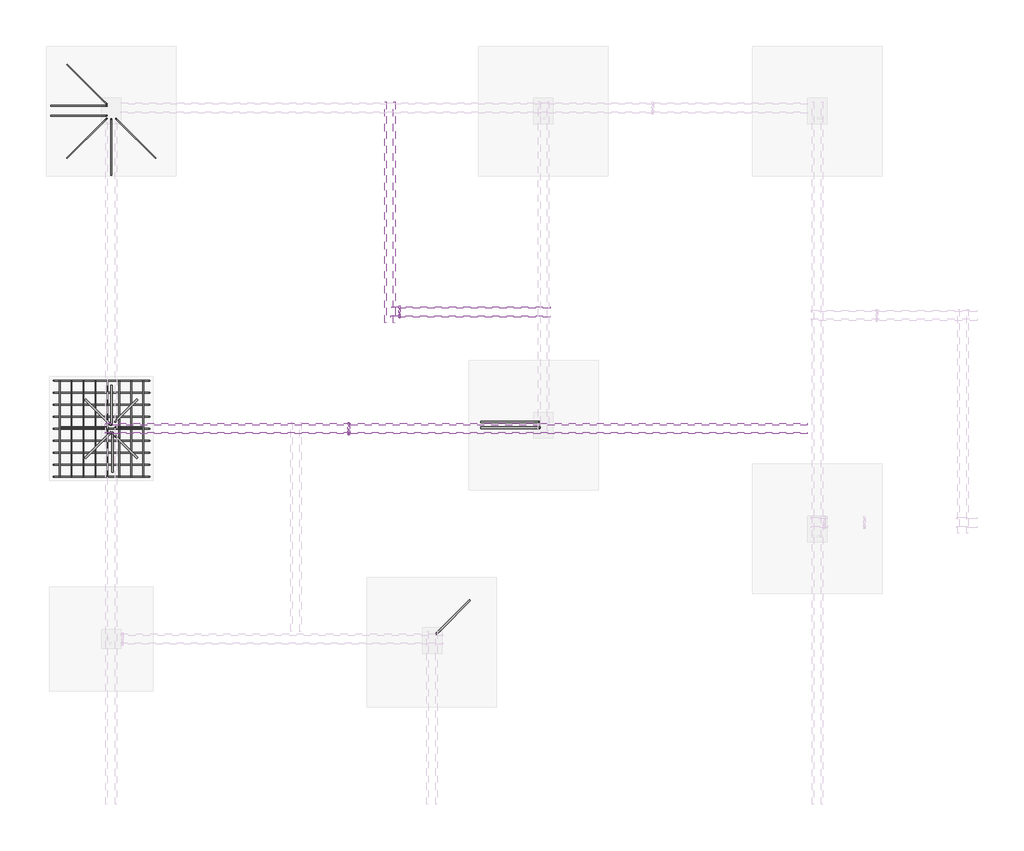
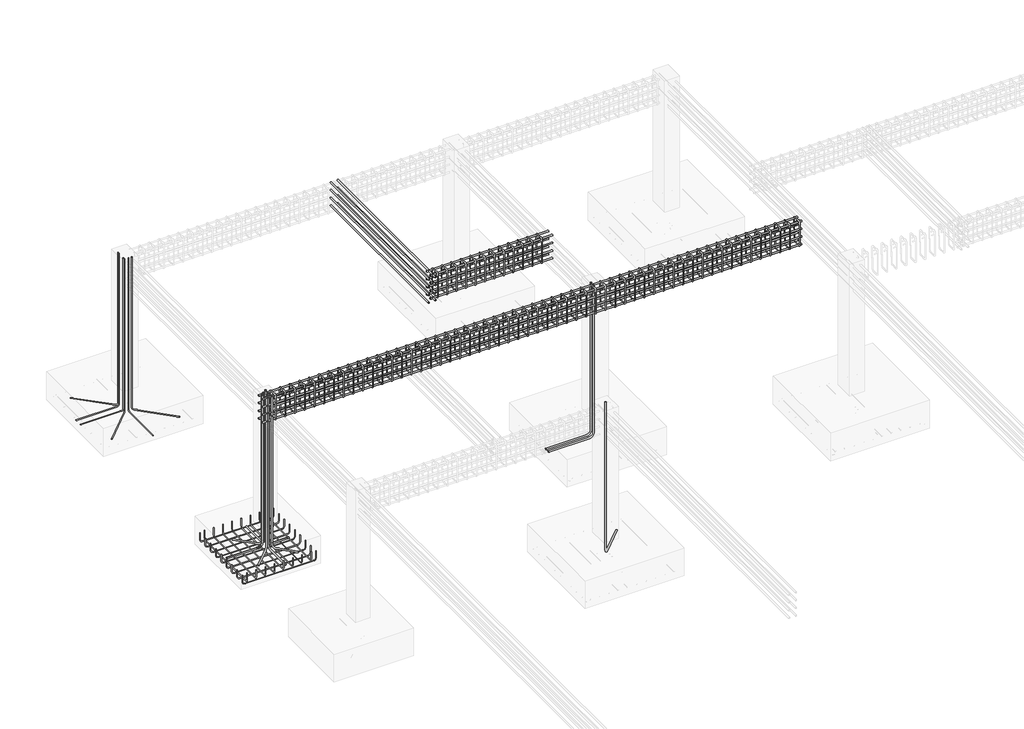
# One storey, part 6 of 10: 28 reinforcing bars.
"""IFC4 building model written with IfcOpenShell, lengths in millimetres."""

from ifc_helpers import new_model, si_unit, point, frame, origin, place, context, project, spatial, polyline, circle_curve, trimmed, segment, composite_curve, source, transform, mapped, element, save
from ifc_brep_helpers import swept_disk

model = new_model("IFC4")

# Units and contexts
model_context = context("Model", 3, world=origin())
ifc_project = project(units=[si_unit("LENGTHUNIT", "METRE", prefix="MILLI")], contexts=[model_context])

# Site, building, storey
site = spatial("IfcSite", under=ifc_project)
building = spatial("IfcBuilding", under=site)
storey = spatial("IfcBuildingStorey", under=building, Elevation=-2133.6)

# Reinforcing bars
placement = place(None, origin())
reinforcing_bar_shape = source(origin(), model_context, "Body", "SolidModel", [
    swept_disk(composite_curve([segment(polyline([(-4484.7164362, 8981.8219177, -2393.6), (-4484.7164362, 8981.8219177, -2504.1)]), True, "CONTINUOUS"), segment(trimmed(circle_curve(frame((-4519.4664362, 8981.8219177, -2504.1), z_axis=(0.0, 1.0, 0.0), x_axis=(34.75, 0.0, 0.0)), 34.75), [point((-4484.7164362, 8981.8219177, -2504.1))], [point((-4519.4664362, 8981.8219177, -2538.85))], True, "CARTESIAN"), True, "CONTINUOUS"), segment(polyline([(-4519.4664362, 8981.8219177, -2538.85), (-5579.6664362, 8981.8219177, -2538.85)]), True, "CONTINUOUS"), segment(trimmed(circle_curve(frame((-5579.6664362, 8981.8219177, -2504.1), z_axis=(0.0, 1.0, 0.0), x_axis=(0.0, 0.0, -34.75)), 34.75), [point((-5579.6664362, 8981.8219177, -2538.85))], [point((-5614.4164362, 8981.8219177, -2504.1))], True, "CARTESIAN"), True, "CONTINUOUS"), segment(polyline([(-5614.4164362, 8981.8219177, -2504.1), (-5614.4164362, 8981.8219177, -2393.6)]), True, "CONTINUOUS")], self_intersect=False), 4.75),
])
element("IfcReinforcingBar", 1, at=placement, inside=storey, context=model_context, shape_type="MappedRepresentation", body=[
    mapped(reinforcing_bar_shape, transform((0.0, 0.0, 0.0), x_axis=(1.0, 0.0, 0.0), y_axis=(0.0, 1.0, 0.0), z_axis=(0.0, 0.0, 1.0))),
    mapped(reinforcing_bar_shape, transform((0.0, -141.2125, 0.0), x_axis=(1.0, 0.0, 0.0), y_axis=(0.0, 1.0, 0.0), z_axis=(0.0, 0.0, 1.0))),
    mapped(reinforcing_bar_shape, transform((0.0, -282.425, 0.0), x_axis=(1.0, 0.0, 0.0), y_axis=(0.0, 1.0, 0.0), z_axis=(0.0, 0.0, 1.0))),
    mapped(reinforcing_bar_shape, transform((0.0, -423.6375, 0.0), x_axis=(1.0, 0.0, 0.0), y_axis=(0.0, 1.0, 0.0), z_axis=(0.0, 0.0, 1.0))),
    mapped(reinforcing_bar_shape, transform((0.0, -564.85, 0.0), x_axis=(1.0, 0.0, 0.0), y_axis=(0.0, 1.0, 0.0), z_axis=(0.0, 0.0, 1.0))),
    mapped(reinforcing_bar_shape, transform((0.0, -706.0625, 0.0), x_axis=(1.0, 0.0, 0.0), y_axis=(0.0, 1.0, 0.0), z_axis=(0.0, 0.0, 1.0))),
    mapped(reinforcing_bar_shape, transform((0.0, -847.275, 0.0), x_axis=(1.0, 0.0, 0.0), y_axis=(0.0, 1.0, 0.0), z_axis=(0.0, 0.0, 1.0))),
    mapped(reinforcing_bar_shape, transform((0.0, -988.4875, 0.0), x_axis=(1.0, 0.0, 0.0), y_axis=(0.0, 1.0, 0.0), z_axis=(0.0, 0.0, 1.0))),
    mapped(reinforcing_bar_shape, transform((0.0, -1129.7, 0.0), x_axis=(1.0, 0.0, 0.0), y_axis=(0.0, 1.0, 0.0), z_axis=(0.0, 0.0, 1.0))),
])
reinforcing_bar_2_shape = source(origin(), model_context, "Body", "SolidModel", [
    swept_disk(composite_curve([segment(polyline([(-4559.6743867, 7852.1219177, -2379.223371), (-4559.6743867, 7852.1219177, -2489.723371)]), True, "CONTINUOUS"), segment(trimmed(circle_curve(frame((-4559.6743867, 7886.8719177, -2489.723371), z_axis=(1.0, 0.0, 0.0), x_axis=(0.0, -34.75, 0.0)), 34.75), [point((-4559.6743867, 7852.1219177, -2489.723371))], [point((-4559.6743867, 7886.8719177, -2524.473371))], True, "CARTESIAN"), True, "CONTINUOUS"), segment(polyline([(-4559.6743867, 7886.8719177, -2524.473371), (-4559.6743867, 8947.0719177, -2524.473371)]), True, "CONTINUOUS"), segment(trimmed(circle_curve(frame((-4559.6743867, 8947.0719177, -2489.723371), z_axis=(1.0, 0.0, 0.0), x_axis=(0.0, 0.0, -34.75)), 34.75), [point((-4559.6743867, 8947.0719177, -2524.473371))], [point((-4559.6743867, 8981.8219177, -2489.723371))], True, "CARTESIAN"), True, "CONTINUOUS"), segment(polyline([(-4559.6743867, 8981.8219177, -2489.723371), (-4559.6743867, 8981.8219177, -2379.223371)]), True, "CONTINUOUS")], self_intersect=False), 4.75),
])
element("IfcReinforcingBar", 2, at=placement, inside=storey, context=model_context, shape_type="MappedRepresentation", body=[
    mapped(reinforcing_bar_2_shape, transform((0.0, 0.0, 0.0), x_axis=(1.0, 0.0, 0.0), y_axis=(0.0, 1.0, 0.0), z_axis=(0.0, 0.0, 1.0))),
    mapped(reinforcing_bar_2_shape, transform((-140.5079612, 0.0, 0.0), x_axis=(1.0, 0.0, 0.0), y_axis=(0.0, 1.0, 0.0), z_axis=(0.0, 0.0, 1.0))),
    mapped(reinforcing_bar_2_shape, transform((-281.0159224, 0.0, 0.0), x_axis=(1.0, 0.0, 0.0), y_axis=(0.0, 1.0, 0.0), z_axis=(0.0, 0.0, 1.0))),
    mapped(reinforcing_bar_2_shape, transform((-421.5238836, 0.0, 0.0), x_axis=(1.0, 0.0, 0.0), y_axis=(0.0, 1.0, 0.0), z_axis=(0.0, 0.0, 1.0))),
    mapped(reinforcing_bar_2_shape, transform((-562.0318448, 0.0, 0.0), x_axis=(1.0, 0.0, 0.0), y_axis=(0.0, 1.0, 0.0), z_axis=(0.0, 0.0, 1.0))),
    mapped(reinforcing_bar_2_shape, transform((-702.539806, 0.0, 0.0), x_axis=(1.0, 0.0, 0.0), y_axis=(0.0, 1.0, 0.0), z_axis=(0.0, 0.0, 1.0))),
    mapped(reinforcing_bar_2_shape, transform((-843.0477672, 0.0, 0.0), x_axis=(1.0, 0.0, 0.0), y_axis=(0.0, 1.0, 0.0), z_axis=(0.0, 0.0, 1.0))),
    mapped(reinforcing_bar_2_shape, transform((-983.5557284, 0.0, 0.0), x_axis=(1.0, 0.0, 0.0), y_axis=(0.0, 1.0, 0.0), z_axis=(0.0, 0.0, 1.0))),
])
element("IfcReinforcingBar", 3, at=placement, inside=storey, context=model_context, shape_type="SolidModel", body=[
    swept_disk(composite_curve([segment(polyline([(-4880.7190942, 12064.1455908, -40.0), (-4880.7190942, 12064.1455908, -2478.85)]), True, "CONTINUOUS"), segment(trimmed(circle_curve(frame((-4856.1471335, 12039.5736302, -2478.85), z_axis=(-0.7071067811865476, -0.7071067811865475, 0.0), x_axis=(-24.57196070000009, 24.57196060000024, 0.0)), 34.75), [point((-4880.7190942, 12064.1455908, -2478.85))], [point((-4856.1471335, 12039.5736302, -2513.6))], True, "CARTESIAN"), True, "CONTINUOUS"), segment(polyline([(-4856.1471335, 12039.5736302, -2513.6), (-4415.8298614, 11599.256358, -2513.6)]), True, "CONTINUOUS")], self_intersect=False), 4.75),
])
element("IfcReinforcingBar", 4, at=placement, inside=storey, context=model_context, shape_type="SolidModel", body=[
    swept_disk(composite_curve([segment(polyline([(-4989.8137781, 12064.1455908, -40.0), (-4989.8137781, 12064.1455908, -2478.85)]), True, "CONTINUOUS"), segment(trimmed(circle_curve(frame((-5014.3857388, 12039.5736302, -2478.85), z_axis=(-0.7071067811865476, 0.7071067811865475, 0.0), x_axis=(24.57196070000009, 24.57196060000024, 0.0)), 34.75), [point((-4989.8137781, 12064.1455908, -2478.85))], [point((-5014.3857388, 12039.5736302, -2513.6))], True, "CARTESIAN"), True, "CONTINUOUS"), segment(polyline([(-5014.3857388, 12039.5736302, -2513.6), (-5454.7030109, 11599.256358, -2513.6)]), True, "CONTINUOUS")], self_intersect=False), 4.75),
])
element("IfcReinforcingBar", 5, at=placement, inside=storey, context=model_context, shape_type="SolidModel", body=[
    swept_disk(composite_curve([segment(polyline([(-4989.8137781, 12237.3982446, -40.0), (-4989.8137781, 12237.3982446, -2478.85)]), True, "CONTINUOUS"), segment(trimmed(circle_curve(frame((-5014.3857388, 12261.9702053, -2478.85), z_axis=(0.7071067811865476, 0.7071067811865475, 0.0), x_axis=(24.57196070000009, -24.57196069999918, 0.0)), 34.75), [point((-4989.8137781, 12237.3982446, -2478.85))], [point((-5014.3857388, 12261.9702053, -2513.6))], True, "CARTESIAN"), True, "CONTINUOUS"), segment(polyline([(-5014.3857388, 12261.9702053, -2513.6), (-5454.7030109, 12702.2874774, -2513.6)]), True, "CONTINUOUS")], self_intersect=False), 4.75),
])
reinforcing_bar_3_shape = source(origin(), model_context, "Body", "SolidModel", [
    swept_disk(composite_curve([segment(polyline([(-4989.8137781, 12214.7595351, -40.0), (-4989.8137781, 12214.7595351, -2478.85)]), True, "CONTINUOUS"), segment(trimmed(circle_curve(frame((-5024.5637781, 12214.7595351, -2478.85), z_axis=(0.0, 1.0, 0.0), x_axis=(34.75, 0.0, 0.0)), 34.75), [point((-4989.8137781, 12214.7595351, -2478.85))], [point((-5024.5637781, 12214.7595351, -2513.6))], True, "CARTESIAN"), True, "CONTINUOUS"), segment(polyline([(-5024.5637781, 12214.7595351, -2513.6), (-5647.2664362, 12214.7595351, -2513.6)]), True, "CONTINUOUS")], self_intersect=False), 4.75),
])
element("IfcReinforcingBar", 6, at=placement, inside=storey, context=model_context, shape_type="MappedRepresentation", body=[
    mapped(reinforcing_bar_3_shape, transform((0.0, 0.0, 0.0), x_axis=(1.0, 0.0, 0.0), y_axis=(0.0, 1.0, 0.0), z_axis=(0.0, 0.0, 1.0))),
    mapped(reinforcing_bar_3_shape, transform((0.0, -114.7595265, 0.0), x_axis=(1.0, 0.0, 0.0), y_axis=(0.0, 1.0, 0.0), z_axis=(0.0, 0.0, 1.0))),
])
element("IfcReinforcingBar", 7, at=placement, inside=storey, context=model_context, shape_type="SolidModel", body=[
    swept_disk(composite_curve([segment(polyline([(-4935.2664362, 12059.1455908, -40.0), (-4935.2664362, 12059.1455908, -2478.85)]), True, "CONTINUOUS"), segment(trimmed(circle_curve(frame((-4935.2664362, 12024.3955908, -2478.85), z_axis=(-1.0, 0.0, 0.0), x_axis=(0.0, 34.75, 0.0)), 34.75), [point((-4935.2664362, 12059.1455908, -2478.85))], [point((-4935.2664362, 12024.3955908, -2513.6))], True, "CARTESIAN"), True, "CONTINUOUS"), segment(polyline([(-4935.2664362, 12024.3955908, -2513.6), (-4935.2664362, 11401.6929328, -2513.6)]), True, "CONTINUOUS")], self_intersect=False), 4.75),
])
element("IfcReinforcingBar", 8, at=placement, inside=storey, context=model_context, shape_type="SolidModel", body=[
    swept_disk(composite_curve([segment(polyline([(103.8835638, 8496.2552961, -40.0), (103.8835638, 8496.2552961, -2426.55)]), True, "CONTINUOUS"), segment(trimmed(circle_curve(frame((36.8335638, 8496.2552961, -2426.55), z_axis=(0.0, 1.0, 0.0), x_axis=(67.05000000000001, 0.0, 0.0)), 67.05), [point((103.8835638, 8496.2552961, -2426.55))], [point((36.8335638, 8496.2552961, -2493.6))], True, "CARTESIAN"), True, "CONTINUOUS"), segment(polyline([(36.8335638, 8496.2552961, -2493.6), (-590.4164362, 8496.2552961, -2493.6)]), True, "CONTINUOUS")], self_intersect=False), 9.55),
])
element("IfcReinforcingBar", 9, at=placement, inside=storey, context=model_context, shape_type="SolidModel", body=[
    swept_disk(composite_curve([segment(polyline([(103.8835638, 8429.1170998, -40.0), (103.8835638, 8429.1170998, -2426.55)]), True, "CONTINUOUS"), segment(trimmed(circle_curve(frame((36.8335638, 8429.1170998, -2426.55), z_axis=(0.0, 1.0, 0.0), x_axis=(67.05000000000001, 0.0, 0.0)), 67.05), [point((103.8835638, 8429.1170998, -2426.55))], [point((36.8335638, 8429.1170998, -2493.6))], True, "CARTESIAN"), True, "CONTINUOUS"), segment(polyline([(36.8335638, 8429.1170998, -2493.6), (-590.4164362, 8429.1170998, -2493.6)]), True, "CONTINUOUS")], self_intersect=False), 9.55),
])
element("IfcReinforcingBar", 10, at=placement, inside=storey, context=model_context, shape_type="SolidModel", body=[
    swept_disk(composite_curve([segment(polyline([(-4944.3664362, 8465.0552961, -40.0), (-4944.3664362, 8465.0552961, -2426.55)]), True, "CONTINUOUS"), segment(trimmed(circle_curve(frame((-4991.7779458, 8512.4668058, -2426.55), z_axis=(0.7071067811865519, 0.7071067811865431, 0.0), x_axis=(47.4115096000005, -47.41150970000126, 0.0)), 67.05), [point((-4944.3664362, 8465.0552961, -2426.55))], [point((-4991.7779458, 8512.4668058, -2493.6))], True, "CARTESIAN"), True, "CONTINUOUS"), segment(polyline([(-4991.7779458, 8512.4668058, -2493.6), (-5240.1883692, 8760.8772292, -2493.6)]), True, "CONTINUOUS")], self_intersect=False), 9.55),
])
element("IfcReinforcingBar", 11, at=placement, inside=storey, context=model_context, shape_type="SolidModel", body=[
    swept_disk(composite_curve([segment(polyline([(-4886.9664362, 8503.1552961, -40.0), (-4886.9664362, 8503.1552961, -2426.55)]), True, "CONTINUOUS"), segment(trimmed(circle_curve(frame((-4839.5549265, 8550.5668058, -2426.55), z_axis=(0.7071067811865519, -0.7071067811865431, 0.0), x_axis=(-47.41150970000035, -47.41150969999944, 0.0)), 67.05), [point((-4886.9664362, 8503.1552961, -2426.55))], [point((-4839.5549265, 8550.5668058, -2493.6))], True, "CARTESIAN"), True, "CONTINUOUS"), segment(polyline([(-4839.5549265, 8550.5668058, -2493.6), (-4629.2445031, 8760.8772292, -2493.6)]), True, "CONTINUOUS")], self_intersect=False), 9.55),
])
element("IfcReinforcingBar", 12, at=placement, inside=storey, context=model_context, shape_type="SolidModel", body=[
    swept_disk(composite_curve([segment(polyline([(-4944.3664362, 8368.8885393, -40.0), (-4944.3664362, 8368.8885393, -2426.55)]), True, "CONTINUOUS"), segment(trimmed(circle_curve(frame((-4991.7779458, 8321.4770296, -2426.55), z_axis=(-0.7071067811865519, 0.7071067811865431, 0.0), x_axis=(47.4115096000005, 47.41150969999944, 0.0)), 67.05), [point((-4944.3664362, 8368.8885393, -2426.55))], [point((-4991.7779458, 8321.4770296, -2493.6))], True, "CARTESIAN"), True, "CONTINUOUS"), segment(polyline([(-4991.7779458, 8321.4770296, -2493.6), (-5240.1883692, 8073.0666062, -2493.6)]), True, "CONTINUOUS")], self_intersect=False), 9.55),
])
element("IfcReinforcingBar", 13, at=placement, inside=storey, context=model_context, shape_type="SolidModel", body=[
    swept_disk(composite_curve([segment(polyline([(-4886.9664362, 8330.7885393, -40.0), (-4886.9664362, 8330.7885393, -2426.55)]), True, "CONTINUOUS"), segment(trimmed(circle_curve(frame((-4839.5549265, 8283.3770296, -2426.55), z_axis=(-0.7071067811865519, -0.7071067811865431, 0.0), x_axis=(-47.41150970000035, 47.41150969999944, 0.0)), 67.05), [point((-4886.9664362, 8330.7885393, -2426.55))], [point((-4839.5549265, 8283.3770296, -2493.6))], True, "CARTESIAN"), True, "CONTINUOUS"), segment(polyline([(-4839.5549265, 8283.3770296, -2493.6), (-4629.2445031, 8073.0666062, -2493.6)]), True, "CONTINUOUS")], self_intersect=False), 9.55),
])
element("IfcReinforcingBar", 14, at=placement, inside=storey, context=model_context, shape_type="SolidModel", body=[
    swept_disk(composite_curve([segment(polyline([(-4933.5805145, 8465.0552961, -40.0), (-4933.5805145, 8465.0552961, -2426.55)]), True, "CONTINUOUS"), segment(trimmed(circle_curve(frame((-4933.5805145, 8532.1052961, -2426.55), z_axis=(1.0, 0.0, 0.0), x_axis=(0.0, -67.05000000000109, 0.0)), 67.05), [point((-4933.5805145, 8465.0552961, -2426.55))], [point((-4933.5805145, 8532.1052961, -2493.6))], True, "CARTESIAN"), True, "CONTINUOUS"), segment(polyline([(-4933.5805145, 8532.1052961, -2493.6), (-4933.5805145, 8930.7552961, -2493.6)]), True, "CONTINUOUS")], self_intersect=False), 9.55),
])
element("IfcReinforcingBar", 15, at=placement, inside=storey, context=model_context, shape_type="SolidModel", body=[
    swept_disk(composite_curve([segment(polyline([(-4923.5805145, 8368.8885393, -40.0), (-4923.5805145, 8368.8885393, -2426.55)]), True, "CONTINUOUS"), segment(trimmed(circle_curve(frame((-4923.5805145, 8301.8385393, -2426.55), z_axis=(-1.0, 0.0, 0.0), x_axis=(0.0, 67.04999999999927, 0.0)), 67.05), [point((-4923.5805145, 8368.8885393, -2426.55))], [point((-4923.5805145, 8301.8385393, -2493.6))], True, "CARTESIAN"), True, "CONTINUOUS"), segment(polyline([(-4923.5805145, 8301.8385393, -2493.6), (-4923.5805145, 7903.1885393, -2493.6)]), True, "CONTINUOUS")], self_intersect=False), 9.55),
])
element("IfcReinforcingBar", 16, at=placement, inside=storey, context=model_context, shape_type="SolidModel", body=[
    swept_disk(composite_curve([segment(polyline([(-4982.4664362, 8420.0552961, -40.0), (-4982.4664362, 8420.0552961, -2426.55)]), True, "CONTINUOUS"), segment(trimmed(circle_curve(frame((-5049.5164362, 8420.0552961, -2426.55), z_axis=(0.0, 1.0, 0.0), x_axis=(67.04999999999927, 0.0, 0.0)), 67.05), [point((-4982.4664362, 8420.0552961, -2426.55))], [point((-5049.5164362, 8420.0552961, -2493.6))], True, "CARTESIAN"), True, "CONTINUOUS"), segment(polyline([(-5049.5164362, 8420.0552961, -2493.6), (-5524.3664362, 8420.0552961, -2493.6)]), True, "CONTINUOUS")], self_intersect=False), 9.55),
])
element("IfcReinforcingBar", 17, at=placement, inside=storey, context=model_context, shape_type="SolidModel", body=[
    swept_disk(composite_curve([segment(polyline([(-4982.4664362, 8429.1170998, -40.0), (-4982.4664362, 8429.1170998, -2426.55)]), True, "CONTINUOUS"), segment(trimmed(circle_curve(frame((-5049.5164362, 8429.1170998, -2426.55), z_axis=(0.0, 1.0, 0.0), x_axis=(67.04999999999927, 0.0, 0.0)), 67.05), [point((-4982.4664362, 8429.1170998, -2426.55))], [point((-5049.5164362, 8429.1170998, -2493.6))], True, "CARTESIAN"), True, "CONTINUOUS"), segment(polyline([(-5049.5164362, 8429.1170998, -2493.6), (-5524.3664362, 8429.1170998, -2493.6)]), True, "CONTINUOUS")], self_intersect=False), 9.55),
])
element("IfcReinforcingBar", 18, at=placement, inside=storey, context=model_context, shape_type="SolidModel", body=[
    swept_disk(composite_curve([segment(polyline([(-4886.9664362, 8420.0552961, -40.0), (-4886.9664362, 8420.0552961, -2426.55)]), True, "CONTINUOUS"), segment(trimmed(circle_curve(frame((-4819.9164362, 8420.0552961, -2426.55), z_axis=(0.0, -1.0, 0.0), x_axis=(-67.05000000000018, 0.0, 0.0)), 67.05), [point((-4886.9664362, 8420.0552961, -2426.55))], [point((-4819.9164362, 8420.0552961, -2493.6))], True, "CARTESIAN"), True, "CONTINUOUS"), segment(polyline([(-4819.9164362, 8420.0552961, -2493.6), (-4573.6664362, 8420.0552961, -2493.6)]), True, "CONTINUOUS")], self_intersect=False), 9.55),
])
element("IfcReinforcingBar", 19, at=placement, inside=storey, context=model_context, shape_type="SolidModel", body=[
    swept_disk(composite_curve([segment(polyline([(-4886.9664362, 8429.1170998, -40.0), (-4886.9664362, 8429.1170998, -2426.55)]), True, "CONTINUOUS"), segment(trimmed(circle_curve(frame((-4819.9164362, 8429.1170998, -2426.55), z_axis=(0.0, -1.0, 0.0), x_axis=(-67.05000000000018, 0.0, 0.0)), 67.05), [point((-4886.9664362, 8429.1170998, -2426.55))], [point((-4819.9164362, 8429.1170998, -2493.6))], True, "CARTESIAN"), True, "CONTINUOUS"), segment(polyline([(-4819.9164362, 8429.1170998, -2493.6), (-4573.6664362, 8429.1170998, -2493.6)]), True, "CONTINUOUS")], self_intersect=False), 9.55),
])
element("IfcReinforcingBar", 20, at=placement, inside=storey, context=model_context, shape_type="SolidModel", body=[
    swept_disk(composite_curve([segment(polyline([(-1109.9664362, 6006.6552961, -40.0), (-1109.9664362, 6006.6552961, -2426.55)]), True, "CONTINUOUS"), segment(trimmed(circle_curve(frame((-1062.5549265, 6054.0668058, -2426.55), z_axis=(0.7071067811865519, -0.7071067811865431, 0.0), x_axis=(-47.411509700000124, -47.41150970000035, 0.0)), 67.05), [point((-1109.9664362, 6006.6552961, -2426.55))], [point((-1062.5549265, 6054.0668058, -2493.6))], True, "CARTESIAN"), True, "CONTINUOUS"), segment(polyline([(-1062.5549265, 6054.0668058, -2493.6), (-717.9445031, 6398.6772292, -2493.6)]), True, "CONTINUOUS")], self_intersect=False), 9.55),
])
reinforcing_bar_4_shape = source(origin(), model_context, "Body", "SolidModel", [
    swept_disk(composite_curve([segment(polyline([(-4816.2164362, 8447.0786993, -109.4049959), (-4816.2164362, 8389.6728105, -51.9991072)]), True, "CONTINUOUS"), segment(trimmed(circle_curve(frame((-4816.2164362, 8372.1719177, -69.5), z_axis=(1.0, 0.0, 0.0), x_axis=(0.0, 17.500892800000656, 17.500892800000003)), 24.75), [point((-4816.2164362, 8389.6728105, -51.9991072))], [point((-4816.2164362, 8347.4219177, -69.5))], True, "CARTESIAN"), True, "CONTINUOUS"), segment(polyline([(-4816.2164362, 8347.4219177, -69.5), (-4816.2164362, 8347.4219177, -430.5)]), True, "CONTINUOUS"), segment(trimmed(circle_curve(frame((-4816.2164362, 8372.1719177, -430.5), z_axis=(1.0, 0.0, 0.0), x_axis=(0.0, -24.75, 0.0)), 24.75), [point((-4816.2164362, 8347.4219177, -430.5))], [point((-4816.2164362, 8372.1719177, -455.25))], True, "CARTESIAN"), True, "CONTINUOUS"), segment(polyline([(-4816.2164362, 8372.1719177, -455.25), (-4816.2164362, 8461.7719177, -455.25)]), True, "CONTINUOUS"), segment(trimmed(circle_curve(frame((-4816.7890599, 8461.7719177, -430.5066251), z_axis=(0.9997323196529888, 0.0, 0.02313631434032496), x_axis=(0.5726236999998946, 0.0, -24.743374899999992)), 24.75), [point((-4816.2164362, 8461.7719177, -455.25))], [point((-4816.7890599, 8486.5219177, -430.5066251))], True, "CARTESIAN"), True, "CONTINUOUS"), segment(polyline([(-4816.7890599, 8486.5219177, -430.5066251), (-4825.1438124, 8486.5219177, -69.4933749)]), True, "CONTINUOUS"), segment(trimmed(circle_curve(frame((-4825.1438124, 8461.7719177, -69.4933749), z_axis=(0.9997323196529888, 0.0, 0.02313631434032496), x_axis=(0.0, 24.75, 0.0)), 24.75), [point((-4825.1438124, 8486.5219177, -69.4933749))], [point((-4825.7164362, 8461.7719177, -44.75))], True, "CARTESIAN"), True, "CONTINUOUS"), segment(polyline([(-4825.7164362, 8461.7719177, -44.75), (-4825.7164362, 8372.1719177, -44.75)]), True, "CONTINUOUS"), segment(trimmed(circle_curve(frame((-4825.7164362, 8372.1719177, -69.5), z_axis=(1.0, 0.0, 0.0), x_axis=(0.0, 0.0, 24.75)), 24.75), [point((-4825.7164362, 8372.1719177, -44.75))], [point((-4825.7164362, 8354.6710249, -87.0008928))], True, "CARTESIAN"), True, "CONTINUOUS"), segment(polyline([(-4825.7164362, 8354.6710249, -87.0008928), (-4825.7164362, 8412.0769136, -144.4067815)]), True, "CONTINUOUS")], self_intersect=False), 4.75),
])
element("IfcReinforcingBar", 21, at=placement, inside=storey, context=model_context, shape_type="MappedRepresentation", body=[
    mapped(reinforcing_bar_4_shape, transform((0.0, 0.0, 0.0), x_axis=(1.0, 0.0, 0.0), y_axis=(0.0, 1.0, 0.0), z_axis=(0.0, 0.0, 1.0))),
    mapped(reinforcing_bar_4_shape, transform((148.8172337, 0.0, 0.0), x_axis=(1.0, 0.0, 0.0), y_axis=(0.0, 1.0, 0.0), z_axis=(0.0, 0.0, 1.0))),
    mapped(reinforcing_bar_4_shape, transform((297.6344674, 0.0, 0.0), x_axis=(1.0, 0.0, 0.0), y_axis=(0.0, 1.0, 0.0), z_axis=(0.0, 0.0, 1.0))),
    mapped(reinforcing_bar_4_shape, transform((446.4517011, 0.0, 0.0), x_axis=(1.0, 0.0, 0.0), y_axis=(0.0, 1.0, 0.0), z_axis=(0.0, 0.0, 1.0))),
    mapped(reinforcing_bar_4_shape, transform((595.2689349, 0.0, 0.0), x_axis=(1.0, 0.0, 0.0), y_axis=(0.0, 1.0, 0.0), z_axis=(0.0, 0.0, 1.0))),
    mapped(reinforcing_bar_4_shape, transform((744.0861686, 0.0, 0.0), x_axis=(1.0, 0.0, 0.0), y_axis=(0.0, 1.0, 0.0), z_axis=(0.0, 0.0, 1.0))),
    mapped(reinforcing_bar_4_shape, transform((892.9034023, 0.0, 0.0), x_axis=(1.0, 0.0, 0.0), y_axis=(0.0, 1.0, 0.0), z_axis=(0.0, 0.0, 1.0))),
    mapped(reinforcing_bar_4_shape, transform((1041.720636, 0.0, 0.0), x_axis=(1.0, 0.0, 0.0), y_axis=(0.0, 1.0, 0.0), z_axis=(0.0, 0.0, 1.0))),
    mapped(reinforcing_bar_4_shape, transform((1190.5378697, 0.0, 0.0), x_axis=(1.0, 0.0, 0.0), y_axis=(0.0, 1.0, 0.0), z_axis=(0.0, 0.0, 1.0))),
    mapped(reinforcing_bar_4_shape, transform((1339.3551034, 0.0, 0.0), x_axis=(1.0, 0.0, 0.0), y_axis=(0.0, 1.0, 0.0), z_axis=(0.0, 0.0, 1.0))),
    mapped(reinforcing_bar_4_shape, transform((1488.1723371, 0.0, 0.0), x_axis=(1.0, 0.0, 0.0), y_axis=(0.0, 1.0, 0.0), z_axis=(0.0, 0.0, 1.0))),
    mapped(reinforcing_bar_4_shape, transform((1636.9895708, 0.0, 0.0), x_axis=(1.0, 0.0, 0.0), y_axis=(0.0, 1.0, 0.0), z_axis=(0.0, 0.0, 1.0))),
    mapped(reinforcing_bar_4_shape, transform((1785.8068046, 0.0, 0.0), x_axis=(1.0, 0.0, 0.0), y_axis=(0.0, 1.0, 0.0), z_axis=(0.0, 0.0, 1.0))),
    mapped(reinforcing_bar_4_shape, transform((1934.6240383, 0.0, 0.0), x_axis=(1.0, 0.0, 0.0), y_axis=(0.0, 1.0, 0.0), z_axis=(0.0, 0.0, 1.0))),
    mapped(reinforcing_bar_4_shape, transform((2083.441272, 0.0, 0.0), x_axis=(1.0, 0.0, 0.0), y_axis=(0.0, 1.0, 0.0), z_axis=(0.0, 0.0, 1.0))),
    mapped(reinforcing_bar_4_shape, transform((2232.2585057, 0.0, 0.0), x_axis=(1.0, 0.0, 0.0), y_axis=(0.0, 1.0, 0.0), z_axis=(0.0, 0.0, 1.0))),
    mapped(reinforcing_bar_4_shape, transform((2381.0757394, 0.0, 0.0), x_axis=(1.0, 0.0, 0.0), y_axis=(0.0, 1.0, 0.0), z_axis=(0.0, 0.0, 1.0))),
    mapped(reinforcing_bar_4_shape, transform((2529.8929731, 0.0, 0.0), x_axis=(1.0, 0.0, 0.0), y_axis=(0.0, 1.0, 0.0), z_axis=(0.0, 0.0, 1.0))),
    mapped(reinforcing_bar_4_shape, transform((2678.7102068, 0.0, 0.0), x_axis=(1.0, 0.0, 0.0), y_axis=(0.0, 1.0, 0.0), z_axis=(0.0, 0.0, 1.0))),
    mapped(reinforcing_bar_4_shape, transform((2827.5274406, 0.0, 0.0), x_axis=(1.0, 0.0, 0.0), y_axis=(0.0, 1.0, 0.0), z_axis=(0.0, 0.0, 1.0))),
    mapped(reinforcing_bar_4_shape, transform((2976.3446743, 0.0, 0.0), x_axis=(1.0, 0.0, 0.0), y_axis=(0.0, 1.0, 0.0), z_axis=(0.0, 0.0, 1.0))),
    mapped(reinforcing_bar_4_shape, transform((3125.161908, 0.0, 0.0), x_axis=(1.0, 0.0, 0.0), y_axis=(0.0, 1.0, 0.0), z_axis=(0.0, 0.0, 1.0))),
    mapped(reinforcing_bar_4_shape, transform((3273.9791417, 0.0, 0.0), x_axis=(1.0, 0.0, 0.0), y_axis=(0.0, 1.0, 0.0), z_axis=(0.0, 0.0, 1.0))),
    mapped(reinforcing_bar_4_shape, transform((3422.7963754, 0.0, 0.0), x_axis=(1.0, 0.0, 0.0), y_axis=(0.0, 1.0, 0.0), z_axis=(0.0, 0.0, 1.0))),
    mapped(reinforcing_bar_4_shape, transform((3571.6136091, 0.0, 0.0), x_axis=(1.0, 0.0, 0.0), y_axis=(0.0, 1.0, 0.0), z_axis=(0.0, 0.0, 1.0))),
    mapped(reinforcing_bar_4_shape, transform((3720.4308428, 0.0, 0.0), x_axis=(1.0, 0.0, 0.0), y_axis=(0.0, 1.0, 0.0), z_axis=(0.0, 0.0, 1.0))),
    mapped(reinforcing_bar_4_shape, transform((3869.2480766, 0.0, 0.0), x_axis=(1.0, 0.0, 0.0), y_axis=(0.0, 1.0, 0.0), z_axis=(0.0, 0.0, 1.0))),
    mapped(reinforcing_bar_4_shape, transform((4018.0653103, 0.0, 0.0), x_axis=(1.0, 0.0, 0.0), y_axis=(0.0, 1.0, 0.0), z_axis=(0.0, 0.0, 1.0))),
    mapped(reinforcing_bar_4_shape, transform((4166.882544, 0.0, 0.0), x_axis=(1.0, 0.0, 0.0), y_axis=(0.0, 1.0, 0.0), z_axis=(0.0, 0.0, 1.0))),
    mapped(reinforcing_bar_4_shape, transform((4315.6997777, 0.0, 0.0), x_axis=(1.0, 0.0, 0.0), y_axis=(0.0, 1.0, 0.0), z_axis=(0.0, 0.0, 1.0))),
    mapped(reinforcing_bar_4_shape, transform((4464.5170114, 0.0, 0.0), x_axis=(1.0, 0.0, 0.0), y_axis=(0.0, 1.0, 0.0), z_axis=(0.0, 0.0, 1.0))),
    mapped(reinforcing_bar_4_shape, transform((4613.3342451, 0.0, 0.0), x_axis=(1.0, 0.0, 0.0), y_axis=(0.0, 1.0, 0.0), z_axis=(0.0, 0.0, 1.0))),
    mapped(reinforcing_bar_4_shape, transform((4762.1514788, 0.0, 0.0), x_axis=(1.0, 0.0, 0.0), y_axis=(0.0, 1.0, 0.0), z_axis=(0.0, 0.0, 1.0))),
    mapped(reinforcing_bar_4_shape, transform((4910.9687125, 0.0, 0.0), x_axis=(1.0, 0.0, 0.0), y_axis=(0.0, 1.0, 0.0), z_axis=(0.0, 0.0, 1.0))),
    mapped(reinforcing_bar_4_shape, transform((5059.7859463, 0.0, 0.0), x_axis=(1.0, 0.0, 0.0), y_axis=(0.0, 1.0, 0.0), z_axis=(0.0, 0.0, 1.0))),
    mapped(reinforcing_bar_4_shape, transform((5208.60318, 0.0, 0.0), x_axis=(1.0, 0.0, 0.0), y_axis=(0.0, 1.0, 0.0), z_axis=(0.0, 0.0, 1.0))),
    mapped(reinforcing_bar_4_shape, transform((5357.4204137, 0.0, 0.0), x_axis=(1.0, 0.0, 0.0), y_axis=(0.0, 1.0, 0.0), z_axis=(0.0, 0.0, 1.0))),
    mapped(reinforcing_bar_4_shape, transform((5506.2376474, 0.0, 0.0), x_axis=(1.0, 0.0, 0.0), y_axis=(0.0, 1.0, 0.0), z_axis=(0.0, 0.0, 1.0))),
    mapped(reinforcing_bar_4_shape, transform((5655.0548811, 0.0, 0.0), x_axis=(1.0, 0.0, 0.0), y_axis=(0.0, 1.0, 0.0), z_axis=(0.0, 0.0, 1.0))),
    mapped(reinforcing_bar_4_shape, transform((5803.8721148, 0.0, 0.0), x_axis=(1.0, 0.0, 0.0), y_axis=(0.0, 1.0, 0.0), z_axis=(0.0, 0.0, 1.0))),
    mapped(reinforcing_bar_4_shape, transform((5952.6893485, 0.0, 0.0), x_axis=(1.0, 0.0, 0.0), y_axis=(0.0, 1.0, 0.0), z_axis=(0.0, 0.0, 1.0))),
    mapped(reinforcing_bar_4_shape, transform((6101.5065823, 0.0, 0.0), x_axis=(1.0, 0.0, 0.0), y_axis=(0.0, 1.0, 0.0), z_axis=(0.0, 0.0, 1.0))),
    mapped(reinforcing_bar_4_shape, transform((6250.323816, 0.0, 0.0), x_axis=(1.0, 0.0, 0.0), y_axis=(0.0, 1.0, 0.0), z_axis=(0.0, 0.0, 1.0))),
    mapped(reinforcing_bar_4_shape, transform((6399.1410497, 0.0, 0.0), x_axis=(1.0, 0.0, 0.0), y_axis=(0.0, 1.0, 0.0), z_axis=(0.0, 0.0, 1.0))),
    mapped(reinforcing_bar_4_shape, transform((6547.9582834, 0.0, 0.0), x_axis=(1.0, 0.0, 0.0), y_axis=(0.0, 1.0, 0.0), z_axis=(0.0, 0.0, 1.0))),
    mapped(reinforcing_bar_4_shape, transform((6696.7755171, 0.0, 0.0), x_axis=(1.0, 0.0, 0.0), y_axis=(0.0, 1.0, 0.0), z_axis=(0.0, 0.0, 1.0))),
    mapped(reinforcing_bar_4_shape, transform((6845.5927508, 0.0, 0.0), x_axis=(1.0, 0.0, 0.0), y_axis=(0.0, 1.0, 0.0), z_axis=(0.0, 0.0, 1.0))),
    mapped(reinforcing_bar_4_shape, transform((6994.4099845, 0.0, 0.0), x_axis=(1.0, 0.0, 0.0), y_axis=(0.0, 1.0, 0.0), z_axis=(0.0, 0.0, 1.0))),
    mapped(reinforcing_bar_4_shape, transform((7143.2272183, 0.0, 0.0), x_axis=(1.0, 0.0, 0.0), y_axis=(0.0, 1.0, 0.0), z_axis=(0.0, 0.0, 1.0))),
    mapped(reinforcing_bar_4_shape, transform((7292.044452, 0.0, 0.0), x_axis=(1.0, 0.0, 0.0), y_axis=(0.0, 1.0, 0.0), z_axis=(0.0, 0.0, 1.0))),
    mapped(reinforcing_bar_4_shape, transform((7440.8616857, 0.0, 0.0), x_axis=(1.0, 0.0, 0.0), y_axis=(0.0, 1.0, 0.0), z_axis=(0.0, 0.0, 1.0))),
    mapped(reinforcing_bar_4_shape, transform((7589.6789194, 0.0, 0.0), x_axis=(1.0, 0.0, 0.0), y_axis=(0.0, 1.0, 0.0), z_axis=(0.0, 0.0, 1.0))),
    mapped(reinforcing_bar_4_shape, transform((7738.4961531, 0.0, 0.0), x_axis=(1.0, 0.0, 0.0), y_axis=(0.0, 1.0, 0.0), z_axis=(0.0, 0.0, 1.0))),
    mapped(reinforcing_bar_4_shape, transform((7887.3133868, 0.0, 0.0), x_axis=(1.0, 0.0, 0.0), y_axis=(0.0, 1.0, 0.0), z_axis=(0.0, 0.0, 1.0))),
    mapped(reinforcing_bar_4_shape, transform((8036.1306205, 0.0, 0.0), x_axis=(1.0, 0.0, 0.0), y_axis=(0.0, 1.0, 0.0), z_axis=(0.0, 0.0, 1.0))),
])
reinforcing_bar_5_shape = source(origin(), model_context, "Body", "SolidModel", [
    swept_disk(composite_curve([segment(polyline([(-5009.5664362, 8364.7826519, -62.1107341), (3253.5989804, 8364.7826519, -62.1107341)]), True, "CONTINUOUS")], self_intersect=False), 9.55),
])
element("IfcReinforcingBar", 22, at=placement, inside=storey, context=model_context, shape_type="MappedRepresentation", body=[
    mapped(reinforcing_bar_5_shape, transform((0.0, 0.0, 0.0), x_axis=(1.0, 0.0, 0.0), y_axis=(0.0, 1.0, 0.0), z_axis=(0.0, 0.0, 1.0))),
    mapped(reinforcing_bar_5_shape, transform((0.0, 0.0, -125.2595106), x_axis=(1.0, 0.0, 0.0), y_axis=(0.0, 1.0, 0.0), z_axis=(0.0, 0.0, 1.0))),
    mapped(reinforcing_bar_5_shape, transform((0.0, 0.0, -250.5190212), x_axis=(1.0, 0.0, 0.0), y_axis=(0.0, 1.0, 0.0), z_axis=(0.0, 0.0, 1.0))),
    mapped(reinforcing_bar_5_shape, transform((0.0, 0.0, -375.7785317), x_axis=(1.0, 0.0, 0.0), y_axis=(0.0, 1.0, 0.0), z_axis=(0.0, 0.0, 1.0))),
])
reinforcing_bar_6_shape = source(origin(), model_context, "Body", "SolidModel", [
    swept_disk(composite_curve([segment(polyline([(-5009.5664362, 8469.1611836, -62.1107341), (3252.5544813, 8469.1611836, -62.1107341)]), True, "CONTINUOUS")], self_intersect=False), 9.55),
])
element("IfcReinforcingBar", 23, at=placement, inside=storey, context=model_context, shape_type="MappedRepresentation", body=[
    mapped(reinforcing_bar_6_shape, transform((0.0, 0.0, 0.0), x_axis=(1.0, 0.0, 0.0), y_axis=(0.0, 1.0, 0.0), z_axis=(0.0, 0.0, 1.0))),
    mapped(reinforcing_bar_6_shape, transform((0.0, 0.0, -125.2595106), x_axis=(1.0, 0.0, 0.0), y_axis=(0.0, 1.0, 0.0), z_axis=(0.0, 0.0, 1.0))),
    mapped(reinforcing_bar_6_shape, transform((0.0, 0.0, -250.5190212), x_axis=(1.0, 0.0, 0.0), y_axis=(0.0, 1.0, 0.0), z_axis=(0.0, 0.0, 1.0))),
    mapped(reinforcing_bar_6_shape, transform((0.0, 0.0, -375.7785317), x_axis=(1.0, 0.0, 0.0), y_axis=(0.0, 1.0, 0.0), z_axis=(0.0, 0.0, 1.0))),
])
reinforcing_bar_7_shape = source(origin(), model_context, "Body", "SolidModel", [
    swept_disk(composite_curve([segment(polyline([(-1710.855702, 12263.1719177, -62.1107341), (-1710.855702, 9664.2065011, -62.1107341)]), True, "CONTINUOUS")], self_intersect=False), 9.55),
])
element("IfcReinforcingBar", 24, at=placement, inside=storey, context=model_context, shape_type="MappedRepresentation", body=[
    mapped(reinforcing_bar_7_shape, transform((0.0, 0.0, 0.0), x_axis=(1.0, 0.0, 0.0), y_axis=(0.0, 1.0, 0.0), z_axis=(0.0, 0.0, 1.0))),
    mapped(reinforcing_bar_7_shape, transform((0.0, 0.0, -125.2595106), x_axis=(1.0, 0.0, 0.0), y_axis=(0.0, 1.0, 0.0), z_axis=(0.0, 0.0, 1.0))),
    mapped(reinforcing_bar_7_shape, transform((0.0, 0.0, -250.5190212), x_axis=(1.0, 0.0, 0.0), y_axis=(0.0, 1.0, 0.0), z_axis=(0.0, 0.0, 1.0))),
    mapped(reinforcing_bar_7_shape, transform((0.0, 0.0, -375.7785317), x_axis=(1.0, 0.0, 0.0), y_axis=(0.0, 1.0, 0.0), z_axis=(0.0, 0.0, 1.0))),
])
reinforcing_bar_8_shape = source(origin(), model_context, "Body", "SolidModel", [
    swept_disk(composite_curve([segment(polyline([(-1606.4771703, 12263.1719177, -62.1107341), (-1606.4771703, 9665.2510003, -62.1107341)]), True, "CONTINUOUS")], self_intersect=False), 9.55),
])
element("IfcReinforcingBar", 25, at=placement, inside=storey, context=model_context, shape_type="MappedRepresentation", body=[
    mapped(reinforcing_bar_8_shape, transform((0.0, 0.0, 0.0), x_axis=(1.0, 0.0, 0.0), y_axis=(0.0, 1.0, 0.0), z_axis=(0.0, 0.0, 1.0))),
    mapped(reinforcing_bar_8_shape, transform((0.0, 0.0, -125.2595106), x_axis=(1.0, 0.0, 0.0), y_axis=(0.0, 1.0, 0.0), z_axis=(0.0, 0.0, 1.0))),
    mapped(reinforcing_bar_8_shape, transform((0.0, 0.0, -250.5190212), x_axis=(1.0, 0.0, 0.0), y_axis=(0.0, 1.0, 0.0), z_axis=(0.0, 0.0, 1.0))),
    mapped(reinforcing_bar_8_shape, transform((0.0, 0.0, -375.7785317), x_axis=(1.0, 0.0, 0.0), y_axis=(0.0, 1.0, 0.0), z_axis=(0.0, 0.0, 1.0))),
])
reinforcing_bar_9_shape = source(origin(), model_context, "Body", "SolidModel", [
    swept_disk(composite_curve([segment(polyline([(-1539.6164368, 9818.6786993, -109.4049959), (-1539.6164368, 9761.2728105, -51.9991072)]), True, "CONTINUOUS"), segment(trimmed(circle_curve(frame((-1539.6164368, 9743.7719177, -69.5), z_axis=(1.0, 0.0, 0.0), x_axis=(0.0, 17.500892800000656, 17.500892800000003)), 24.75), [point((-1539.6164368, 9761.2728105, -51.9991072))], [point((-1539.6164368, 9719.0219177, -69.5))], True, "CARTESIAN"), True, "CONTINUOUS"), segment(polyline([(-1539.6164368, 9719.0219177, -69.5), (-1539.6164368, 9719.0219177, -430.5)]), True, "CONTINUOUS"), segment(trimmed(circle_curve(frame((-1539.6164368, 9743.7719177, -430.5), z_axis=(1.0, 0.0, 0.0), x_axis=(0.0, -24.75, 0.0)), 24.75), [point((-1539.6164368, 9719.0219177, -430.5))], [point((-1539.6164368, 9743.7719177, -455.25))], True, "CARTESIAN"), True, "CONTINUOUS"), segment(polyline([(-1539.6164368, 9743.7719177, -455.25), (-1539.6164368, 9833.3719177, -455.25)]), True, "CONTINUOUS"), segment(trimmed(circle_curve(frame((-1540.1890606, 9833.3719177, -430.5066251), z_axis=(0.9997323196529888, 0.0, 0.02313631434032496), x_axis=(0.5726237999999739, 0.0, -24.743374899999992)), 24.75), [point((-1539.6164368, 9833.3719177, -455.25))], [point((-1540.1890606, 9858.1219177, -430.5066251))], True, "CARTESIAN"), True, "CONTINUOUS"), segment(polyline([(-1540.1890606, 9858.1219177, -430.5066251), (-1548.543813, 9858.1219177, -69.4933749)]), True, "CONTINUOUS"), segment(trimmed(circle_curve(frame((-1548.543813, 9833.3719177, -69.4933749), z_axis=(0.9997323196529888, 0.0, 0.02313631434032496), x_axis=(0.0, 24.75, 0.0)), 24.75), [point((-1548.543813, 9858.1219177, -69.4933749))], [point((-1549.1164368, 9833.3719177, -44.75))], True, "CARTESIAN"), True, "CONTINUOUS"), segment(polyline([(-1549.1164368, 9833.3719177, -44.75), (-1549.1164368, 9743.7719177, -44.75)]), True, "CONTINUOUS"), segment(trimmed(circle_curve(frame((-1549.1164368, 9743.7719177, -69.5), z_axis=(1.0, 0.0, 0.0), x_axis=(0.0, 0.0, 24.75)), 24.75), [point((-1549.1164368, 9743.7719177, -44.75))], [point((-1549.1164368, 9726.2710249, -87.0008928))], True, "CARTESIAN"), True, "CONTINUOUS"), segment(polyline([(-1549.1164368, 9726.2710249, -87.0008928), (-1549.1164368, 9783.6769136, -144.4067815)]), True, "CONTINUOUS")], self_intersect=False), 4.75),
])
element("IfcReinforcingBar", 26, at=placement, inside=storey, context=model_context, shape_type="MappedRepresentation", body=[
    mapped(reinforcing_bar_9_shape, transform((0.0, 0.0, 0.0), x_axis=(1.0, 0.0, 0.0), y_axis=(0.0, 1.0, 0.0), z_axis=(0.0, 0.0, 1.0))),
    mapped(reinforcing_bar_9_shape, transform((145.3116101, 0.0, 0.0), x_axis=(1.0, 0.0, 0.0), y_axis=(0.0, 1.0, 0.0), z_axis=(0.0, 0.0, 1.0))),
    mapped(reinforcing_bar_9_shape, transform((290.6232203, 0.0, 0.0), x_axis=(1.0, 0.0, 0.0), y_axis=(0.0, 1.0, 0.0), z_axis=(0.0, 0.0, 1.0))),
    mapped(reinforcing_bar_9_shape, transform((435.9348304, 0.0, 0.0), x_axis=(1.0, 0.0, 0.0), y_axis=(0.0, 1.0, 0.0), z_axis=(0.0, 0.0, 1.0))),
    mapped(reinforcing_bar_9_shape, transform((581.2464406, 0.0, 0.0), x_axis=(1.0, 0.0, 0.0), y_axis=(0.0, 1.0, 0.0), z_axis=(0.0, 0.0, 1.0))),
    mapped(reinforcing_bar_9_shape, transform((726.5580507, 0.0, 0.0), x_axis=(1.0, 0.0, 0.0), y_axis=(0.0, 1.0, 0.0), z_axis=(0.0, 0.0, 1.0))),
    mapped(reinforcing_bar_9_shape, transform((871.8696609, 0.0, 0.0), x_axis=(1.0, 0.0, 0.0), y_axis=(0.0, 1.0, 0.0), z_axis=(0.0, 0.0, 1.0))),
    mapped(reinforcing_bar_9_shape, transform((1017.181271, 0.0, 0.0), x_axis=(1.0, 0.0, 0.0), y_axis=(0.0, 1.0, 0.0), z_axis=(0.0, 0.0, 1.0))),
    mapped(reinforcing_bar_9_shape, transform((1162.4928811, 0.0, 0.0), x_axis=(1.0, 0.0, 0.0), y_axis=(0.0, 1.0, 0.0), z_axis=(0.0, 0.0, 1.0))),
    mapped(reinforcing_bar_9_shape, transform((1307.8044913, 0.0, 0.0), x_axis=(1.0, 0.0, 0.0), y_axis=(0.0, 1.0, 0.0), z_axis=(0.0, 0.0, 1.0))),
    mapped(reinforcing_bar_9_shape, transform((1453.1161014, 0.0, 0.0), x_axis=(1.0, 0.0, 0.0), y_axis=(0.0, 1.0, 0.0), z_axis=(0.0, 0.0, 1.0))),
    mapped(reinforcing_bar_9_shape, transform((1598.4277116, 0.0, 0.0), x_axis=(1.0, 0.0, 0.0), y_axis=(0.0, 1.0, 0.0), z_axis=(0.0, 0.0, 1.0))),
])
reinforcing_bar_10_shape = source(origin(), model_context, "Body", "SolidModel", [
    swept_disk(composite_curve([segment(polyline([(-1646.510101, 9736.3826519, -62.1107341), (225.3835638, 9736.3826519, -62.1107341)]), True, "CONTINUOUS")], self_intersect=False), 9.55),
])
element("IfcReinforcingBar", 27, at=placement, inside=storey, context=model_context, shape_type="MappedRepresentation", body=[
    mapped(reinforcing_bar_10_shape, transform((0.0, 0.0, 0.0), x_axis=(1.0, 0.0, 0.0), y_axis=(0.0, 1.0, 0.0), z_axis=(0.0, 0.0, 1.0))),
    mapped(reinforcing_bar_10_shape, transform((0.0, 0.0, -125.2595106), x_axis=(1.0, 0.0, 0.0), y_axis=(0.0, 1.0, 0.0), z_axis=(0.0, 0.0, 1.0))),
    mapped(reinforcing_bar_10_shape, transform((0.0, 0.0, -250.5190212), x_axis=(1.0, 0.0, 0.0), y_axis=(0.0, 1.0, 0.0), z_axis=(0.0, 0.0, 1.0))),
    mapped(reinforcing_bar_10_shape, transform((0.0, 0.0, -375.7785317), x_axis=(1.0, 0.0, 0.0), y_axis=(0.0, 1.0, 0.0), z_axis=(0.0, 0.0, 1.0))),
])
reinforcing_bar_11_shape = source(origin(), model_context, "Body", "SolidModel", [
    swept_disk(composite_curve([segment(polyline([(-1642.3083792, 9840.7611836, -62.1107341), (225.3835638, 9840.7611836, -62.1107341)]), True, "CONTINUOUS")], self_intersect=False), 9.55),
])
element("IfcReinforcingBar", 28, at=placement, inside=storey, context=model_context, shape_type="MappedRepresentation", body=[
    mapped(reinforcing_bar_11_shape, transform((0.0, 0.0, 0.0), x_axis=(1.0, 0.0, 0.0), y_axis=(0.0, 1.0, 0.0), z_axis=(0.0, 0.0, 1.0))),
    mapped(reinforcing_bar_11_shape, transform((0.0, 0.0, -125.2595106), x_axis=(1.0, 0.0, 0.0), y_axis=(0.0, 1.0, 0.0), z_axis=(0.0, 0.0, 1.0))),
    mapped(reinforcing_bar_11_shape, transform((0.0, 0.0, -250.5190212), x_axis=(1.0, 0.0, 0.0), y_axis=(0.0, 1.0, 0.0), z_axis=(0.0, 0.0, 1.0))),
    mapped(reinforcing_bar_11_shape, transform((0.0, 0.0, -375.7785317), x_axis=(1.0, 0.0, 0.0), y_axis=(0.0, 1.0, 0.0), z_axis=(0.0, 0.0, 1.0))),
])

save(model, "model.ifc")

# Revit data of these elements
# Elements 1, 2, 3, 4, 5, 6, 7, 8, 9, 10, 11, 12, 13, 14, 15, 16, 17, 18, 19, 20, 21, 22, 23, 24, 25, 26, 27, 28 (IfcReinforcingBar)
#   Phase Created = New Construction
